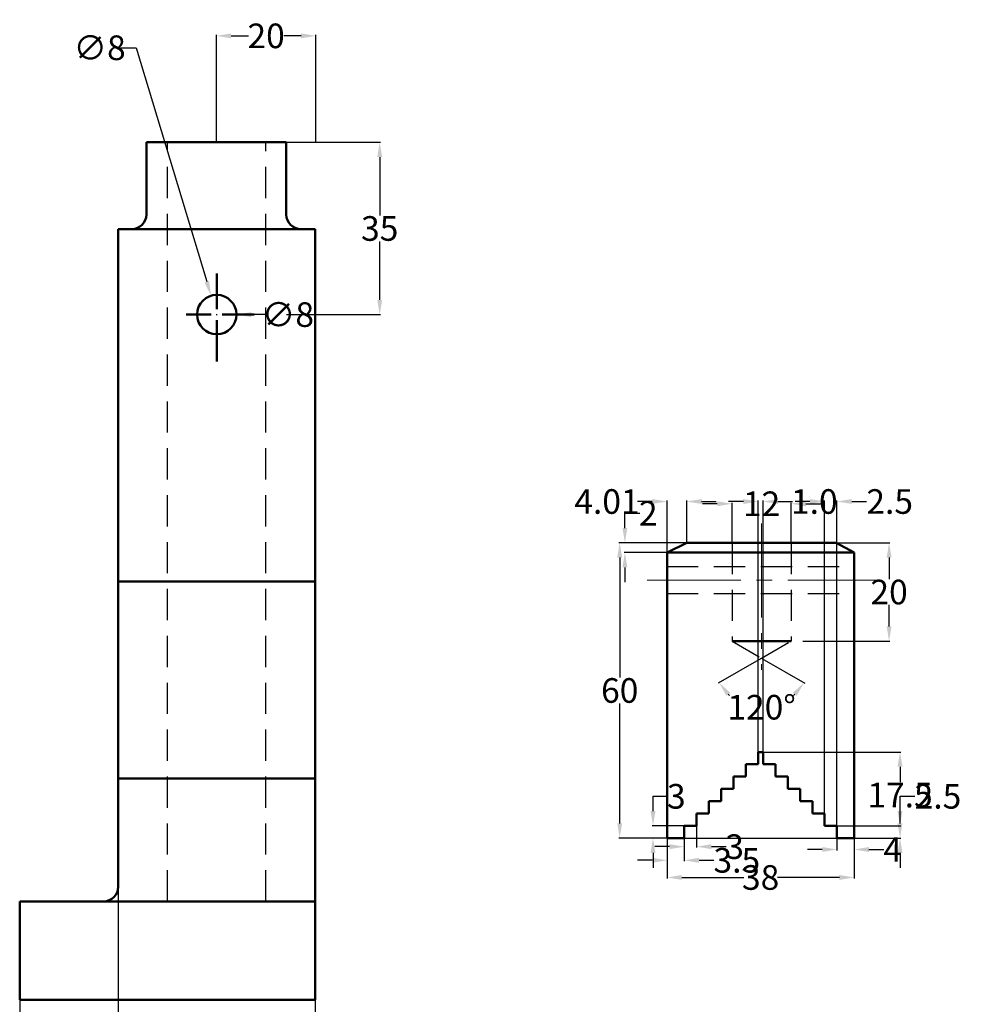
# Model space of a CAD drawing. Units: metres. Extents: x -2793 to -2360, y -31 to 491.
# Tile 4 of 4: x -2552 to -2360, y 144 to 344. Entities that reach past the tile are written whole.
import ezdxf

# ---------------------------------------------------------------- set-up
doc = ezdxf.new("R2010")
doc.units = ezdxf.units.M
doc.linetypes.add('CENTER2', pattern=[28.575, 19.05, -3.175, 3.175, -3.175])
doc.linetypes.add('DASHED2', pattern=[9.525, 6.35, -3.175])
for name, color, linetype, lineweight in [('M-CNTR', 9, 'CENTER2', 18), ('M-DIMS', 2, 'Continuous', 25), ('M-HIDN', 9, 'DASHED2', 25), ('M-OUTL', 7, 'Continuous', 50)]:
    doc.layers.add(name, color=color, linetype=linetype, lineweight=lineweight)
doc.styles.get("Standard").update_dxf_attribs({"font": 'arial.ttf'})
doc.dimstyles.get("Standard").update_dxf_attribs({"dimtxt": 5, "dimasz": 3, "dimexe": 0.18, "dimexo": 0.0625, "dimgap": 0.09, "dimtad": 0, "dimtih": 1, "dimtoh": 1, "dimdec": 0, "dimzin": 0, "dimdsep": 46, "dimtxsty": 'Standard', "dimcen": 0.09, "dimclrd": 254, "dimclre": 254, "dimadec": 0, "dimazin": 0, "dimtfac": 1, "dimtdec": 0, "dimtofl": 0, "dimtmove": 0, "dimatfit": 3, "dimfxl": 1, "dimtolj": 1, "dimtzin": 0, "dimarcsym": 0})

# ---------------------------------------------------------------- blocks, each defined once
blk = doc.blocks.new('*D30')
at = {"layer": 'Defpoints', "color": 0, "transparency": 16777216}
for p in [(-2497.49, 319.4), (-2497.49, 284.4), (-2478.51, 284.4)]:
    blk.add_point(p, dxfattribs=at)
at = {"layer": 'M-DIMS', "color": 0, "lineweight": -2, "transparency": 16777216}
for p, q in [((-2497.43, 319.4), (-2478.33, 319.4)), ((-2478.51, 316.4), (-2478.51, 304.53)), ((-2478.51, 287.4), (-2478.51, 299.27)), ((-2497.43, 284.4), (-2478.33, 284.4))]:
    blk.add_line(p, q, dxfattribs=at)
at = {"layer": 'M-DIMS', "color": 0, "transparency": 16777216}
for points in [[(-2479.01, 316.4), (-2478.01, 316.4), (-2478.51, 319.4)], [(-2479.01, 287.4), (-2478.01, 287.4), (-2478.51, 284.4)]]:
    blk.add_solid(points, dxfattribs=at)
at = {"layer": 'M-DIMS', "color": 0, "transparency": 16777216, "insert": (-2478.51, 301.9), "char_height": 5, "attachment_point": 5}
blk.add_mtext('\\A1;{\\fTimes New Roman|b0|i0|c0|p18;35}', dxfattribs=at)
blk = doc.blocks.new('*D31')
at = {"layer": 'Defpoints', "color": 0, "transparency": 16777216}
for p in [(-2491.47, 341.03), (-2511.68, 319.4), (-2491.47, 319.4)]:
    blk.add_point(p, dxfattribs=at)
at = {"layer": 'M-DIMS', "color": 0, "lineweight": -2, "transparency": 16777216}
for p, q in [((-2511.68, 319.46), (-2511.68, 341.21)), ((-2508.68, 341.03), (-2505.14, 341.03)), ((-2494.47, 341.03), (-2498, 341.03)), ((-2491.47, 319.46), (-2491.47, 341.21))]:
    blk.add_line(p, q, dxfattribs=at)
at = {"layer": 'M-DIMS', "color": 0, "transparency": 16777216}
for points in [[(-2508.68, 341.53), (-2508.68, 340.53), (-2511.68, 341.03)], [(-2494.47, 341.53), (-2494.47, 340.53), (-2491.47, 341.03)]]:
    blk.add_solid(points, dxfattribs=at)
at = {"layer": 'M-DIMS', "color": 0, "transparency": 16777216, "insert": (-2501.57, 341.03), "char_height": 5, "attachment_point": 5}
blk.add_mtext('\\A1;{\\fTimes New Roman|b0|i0|c0|p18;20}', dxfattribs=at)
blk = doc.blocks.new('*D32')
at = {"layer": 'Defpoints', "color": 0, "transparency": 16777216}
for p in [(-2512.76, 288.23), (-2510.45, 280.57)]:
    blk.add_point(p, dxfattribs=at)
at = {"layer": 'M-DIMS', "color": 0, "lineweight": -2, "transparency": 16777216}
for p, q in [((-2531.14, 338.61), (-2527.94, 338.61)), ((-2527.94, 338.61), (-2513.62, 291.1)), ((-2511.7, 284.4), (-2511.52, 284.4)), ((-2511.61, 284.31), (-2511.61, 284.49))]:
    blk.add_line(p, q, dxfattribs=at)
at = {"layer": 'M-DIMS', "color": 0, "transparency": 16777216}
blk.add_solid([(-2513.15, 291.25), (-2514.1, 290.96), (-2512.76, 288.23)], dxfattribs=at)
at = {"layer": 'M-DIMS', "color": 0, "transparency": 16777216, "insert": (-2535.39, 338.61), "char_height": 5, "attachment_point": 5}
blk.add_mtext('\\A1;{\\fTimes New Roman|b0|i0|c0|p18;∅8}', dxfattribs=at)
blk = doc.blocks.new('*D48')
at = {"layer": 'Defpoints', "color": 0, "transparency": 16777216}
for p in [(-2406.98, 218.04), (-2394.98, 218.04), (-2400.98, 214.59), (-2400.98, 214.59), (-2404.39, 205.24)]:
    blk.add_point(p, dxfattribs=at)
at = {"layer": 'M-DIMS', "color": 0, "lineweight": -2, "transparency": 16777216}
for p, q in [((-2401.04, 214.56), (-2409.76, 209.54)), ((-2400.93, 214.56), (-2392.2, 209.54))]:
    blk.add_line(p, q, dxfattribs=at)
for start, end in [(227.2559, 229.3723), (310.6277, 312.7441)]:
    blk.add_arc((-2400.98, 214.59), 9.95, start, end, dxfattribs=at)
at = {"layer": 'M-DIMS', "color": 0, "transparency": 16777216}
for points in [[(-2408.13, 206.97), (-2407.35, 207.59), (-2409.61, 209.63)], [(-2394.62, 207.59), (-2393.84, 206.97), (-2392.36, 209.63)]]:
    blk.add_solid(points, dxfattribs=at)
at = {"layer": 'M-DIMS', "color": 0, "transparency": 16777216, "insert": (-2400.98, 204.64), "char_height": 5, "attachment_point": 5}
blk.add_mtext('\\A1;{\\fTimes New Roman|b0|i0|c0|p18;120°}', dxfattribs=at)
blk = doc.blocks.new('*D49')
at = {"layer": 'Defpoints', "color": 0, "transparency": 16777216}
for p in [(-2392.68, 238.04), (-2392.68, 218.04), (-2375.09, 218.04)]:
    blk.add_point(p, dxfattribs=at)
at = {"layer": 'M-DIMS', "color": 0, "lineweight": -2, "transparency": 16777216}
for p, q in [((-2392.62, 238.04), (-2374.91, 238.04)), ((-2375.09, 235.04), (-2375.09, 230.67)), ((-2375.09, 221.04), (-2375.09, 225.41)), ((-2392.62, 218.04), (-2374.91, 218.04))]:
    blk.add_line(p, q, dxfattribs=at)
at = {"layer": 'M-DIMS', "color": 0, "transparency": 16777216}
for points in [[(-2375.59, 235.04), (-2374.59, 235.04), (-2375.09, 238.04)], [(-2375.59, 221.04), (-2374.59, 221.04), (-2375.09, 218.04)]]:
    blk.add_solid(points, dxfattribs=at)
at = {"layer": 'M-DIMS', "color": 0, "transparency": 16777216, "insert": (-2375.09, 228.04), "char_height": 5, "attachment_point": 5}
blk.add_mtext('\\A1;{\\fTimes New Roman|b0|i0|c0|p18;20}', dxfattribs=at)
blk = doc.blocks.new('*D50')
at = {"layer": 'Defpoints', "color": 0, "transparency": 16777216}
for p in [(-2394.98, 245.97), (-2406.98, 238.04), (-2394.98, 238.04)]:
    blk.add_point(p, dxfattribs=at)
at = {"layer": 'M-DIMS', "color": 0, "lineweight": -2, "transparency": 16777216}
for p, q in [((-2406.98, 238.1), (-2406.98, 246.15)), ((-2394.98, 238.1), (-2394.98, 246.15)), ((-2409.98, 245.97), (-2412.98, 245.97)), ((-2391.98, 245.97), (-2388.98, 245.97))]:
    blk.add_line(p, q, dxfattribs=at)
at = {"layer": 'M-DIMS', "color": 0, "transparency": 16777216}
for points in [[(-2409.98, 246.47), (-2409.98, 245.47), (-2406.98, 245.97)], [(-2391.98, 246.47), (-2391.98, 245.47), (-2394.98, 245.97)]]:
    blk.add_solid(points, dxfattribs=at)
at = {"layer": 'M-DIMS', "color": 0, "transparency": 16777216, "insert": (-2400.98, 245.97), "char_height": 5, "attachment_point": 5}
blk.add_mtext('\\A1;{\\fTimes New Roman|b0|i0|c0|p18;12}', dxfattribs=at)
blk = doc.blocks.new('*D51')
at = {"layer": 'Defpoints', "color": 0, "transparency": 16777216}
for p in [(-2420.83, 238.04), (-2429.78, 178.04), (-2420.17, 178.04)]:
    blk.add_point(p, dxfattribs=at)
at = {"layer": 'M-DIMS', "color": 0, "lineweight": -2, "transparency": 16777216}
for p, q in [((-2420.9, 238.04), (-2429.96, 238.04)), ((-2429.78, 235.04), (-2429.78, 210.67)), ((-2429.78, 181.04), (-2429.78, 205.41)), ((-2420.23, 178.04), (-2429.96, 178.04))]:
    blk.add_line(p, q, dxfattribs=at)
at = {"layer": 'M-DIMS', "color": 0, "transparency": 16777216}
for points in [[(-2430.28, 235.04), (-2429.28, 235.04), (-2429.78, 238.04)], [(-2430.28, 181.04), (-2429.28, 181.04), (-2429.78, 178.04)]]:
    blk.add_solid(points, dxfattribs=at)
at = {"layer": 'M-DIMS', "color": 0, "transparency": 16777216, "insert": (-2429.78, 208.04), "char_height": 5, "attachment_point": 5}
blk.add_mtext('\\A1;{\\fTimes New Roman|b0|i0|c0|p18;60}', dxfattribs=at)
blk = doc.blocks.new('*D52')
at = {"layer": 'Defpoints', "color": 0, "transparency": 16777216}
for p in [(-2423.02, 180.54), (-2416.67, 180.54), (-2416.67, 178.04)]:
    blk.add_point(p, dxfattribs=at)
at = {"layer": 'M-DIMS', "color": 0, "lineweight": -2, "transparency": 16777216}
for p, q in [((-2423.02, 183.54), (-2423.02, 186.54)), ((-2423.02, 186.54), (-2420.02, 186.54)), ((-2416.73, 180.54), (-2423.2, 180.54)), ((-2416.73, 178.04), (-2423.2, 178.04)), ((-2423.02, 175.04), (-2423.02, 172.04))]:
    blk.add_line(p, q, dxfattribs=at)
at = {"layer": 'M-DIMS', "color": 0, "transparency": 16777216}
for points in [[(-2423.52, 183.54), (-2422.52, 183.54), (-2423.02, 180.54)], [(-2423.52, 175.04), (-2422.52, 175.04), (-2423.02, 178.04)]]:
    blk.add_solid(points, dxfattribs=at)
at = {"layer": 'M-DIMS', "color": 0, "transparency": 16777216, "insert": (-2418.29, 186.54), "char_height": 5, "attachment_point": 5}
blk.add_mtext('\\A1;3', dxfattribs=at)
blk = doc.blocks.new('*D53')
at = {"layer": 'Defpoints', "color": 0, "transparency": 16777216}
for p in [(-2416.67, 180.54), (-2414.17, 180.54), (-2414.17, 176.31)]:
    blk.add_point(p, dxfattribs=at)
at = {"layer": 'M-DIMS', "color": 0, "lineweight": -2, "transparency": 16777216}
for p, q in [((-2416.67, 180.48), (-2416.67, 176.13)), ((-2414.17, 180.48), (-2414.17, 176.13)), ((-2419.67, 176.31), (-2422.67, 176.31)), ((-2411.17, 176.31), (-2408.17, 176.31))]:
    blk.add_line(p, q, dxfattribs=at)
at = {"layer": 'M-DIMS', "color": 0, "transparency": 16777216}
for points in [[(-2419.67, 176.81), (-2419.67, 175.81), (-2416.67, 176.31)], [(-2411.17, 176.81), (-2411.17, 175.81), (-2414.17, 176.31)]]:
    blk.add_solid(points, dxfattribs=at)
at = {"layer": 'M-DIMS', "color": 0, "transparency": 16777216, "insert": (-2406.45, 176.31), "char_height": 5, "attachment_point": 5}
blk.add_mtext('\\A1;3', dxfattribs=at)
blk = doc.blocks.new('*D54')
at = {"layer": 'Defpoints', "color": 0, "transparency": 16777216}
for p in [(-2420.17, 178.04), (-2382.17, 178.04), (-2382.17, 170.05)]:
    blk.add_point(p, dxfattribs=at)
at = {"layer": 'M-DIMS', "color": 0, "lineweight": -2, "transparency": 16777216}
for p, q in [((-2420.17, 177.98), (-2420.17, 169.87)), ((-2382.17, 177.98), (-2382.17, 169.87)), ((-2417.17, 170.05), (-2404.59, 170.05)), ((-2385.17, 170.05), (-2397.75, 170.05))]:
    blk.add_line(p, q, dxfattribs=at)
at = {"layer": 'M-DIMS', "color": 0, "transparency": 16777216}
for points in [[(-2417.17, 170.55), (-2417.17, 169.55), (-2420.17, 170.05)], [(-2385.17, 170.55), (-2385.17, 169.55), (-2382.17, 170.05)]]:
    blk.add_solid(points, dxfattribs=at)
at = {"layer": 'M-DIMS', "color": 0, "transparency": 16777216, "insert": (-2401.17, 170.05), "char_height": 5, "attachment_point": 5}
blk.add_mtext('\\A1;{\\fTimes New Roman|b0|i0|c0|p18;38}', dxfattribs=at)
blk = doc.blocks.new('*D55')
at = {"layer": 'Defpoints', "color": 0, "transparency": 16777216}
for p in [(-2385.67, 178.04), (-2382.17, 178.04), (-2382.17, 175.73)]:
    blk.add_point(p, dxfattribs=at)
at = {"layer": 'M-DIMS', "color": 0, "lineweight": -2, "transparency": 16777216}
for p, q in [((-2385.67, 177.98), (-2385.67, 175.55)), ((-2382.17, 177.98), (-2382.17, 175.55)), ((-2388.67, 175.73), (-2391.67, 175.73)), ((-2379.17, 175.73), (-2376.17, 175.73))]:
    blk.add_line(p, q, dxfattribs=at)
at = {"layer": 'M-DIMS', "color": 0, "transparency": 16777216}
for points in [[(-2388.67, 176.23), (-2388.67, 175.23), (-2385.67, 175.73)], [(-2379.17, 176.23), (-2379.17, 175.23), (-2382.17, 175.73)]]:
    blk.add_solid(points, dxfattribs=at)
at = {"layer": 'M-DIMS', "color": 0, "transparency": 16777216, "insert": (-2374.35, 175.73), "char_height": 5, "attachment_point": 5}
blk.add_mtext('\\A1;4', dxfattribs=at)
blk = doc.blocks.new('*D58')
at = {"layer": 'Defpoints', "color": 0, "transparency": 16777216}
for p in [(-2531.61, 168.18), (-2551.61, 165.18), (-2531.61, 121.23)]:
    blk.add_point(p, dxfattribs=at)
at = {"layer": 'M-DIMS', "color": 254, "lineweight": -2, "transparency": 16777216}
for p, q in [((-2531.61, 168.11), (-2531.61, 121.05)), ((-2551.61, 165.11), (-2551.61, 121.05)), ((-2548.61, 121.23), (-2545.31, 121.23)), ((-2534.61, 121.23), (-2537.9, 121.23))]:
    blk.add_line(p, q, dxfattribs=at)
at = {"layer": 'M-DIMS', "color": 254, "transparency": 16777216}
for points in [[(-2548.61, 121.73), (-2548.61, 120.73), (-2551.61, 121.23)], [(-2534.61, 121.73), (-2534.61, 120.73), (-2531.61, 121.23)]]:
    blk.add_solid(points, dxfattribs=at)
at = {"layer": 'M-DIMS', "color": 0, "transparency": 16777216, "insert": (-2541.61, 121.23), "char_height": 5, "attachment_point": 5}
blk.add_mtext('\\A1;20', dxfattribs=at)
blk = doc.blocks.new('*D59')
at = {"layer": 'Defpoints', "color": 0, "transparency": 16777216}
for p in [(-2531.61, 168.18), (-2491.61, 145.18), (-2491.61, 121.23)]:
    blk.add_point(p, dxfattribs=at)
at = {"layer": 'M-DIMS', "color": 254, "lineweight": -2, "transparency": 16777216}
for p, q in [((-2531.61, 168.11), (-2531.61, 121.05)), ((-2491.61, 145.11), (-2491.61, 121.05)), ((-2528.61, 121.23), (-2515.37, 121.23)), ((-2494.61, 121.23), (-2507.84, 121.23))]:
    blk.add_line(p, q, dxfattribs=at)
at = {"layer": 'M-DIMS', "color": 254, "transparency": 16777216}
for points in [[(-2528.61, 121.73), (-2528.61, 120.73), (-2531.61, 121.23)], [(-2494.61, 121.73), (-2494.61, 120.73), (-2491.61, 121.23)]]:
    blk.add_solid(points, dxfattribs=at)
at = {"layer": 'M-DIMS', "color": 0, "transparency": 16777216, "insert": (-2511.61, 121.23), "char_height": 5, "attachment_point": 5}
blk.add_mtext('\\A1;40', dxfattribs=at)
blk = doc.blocks.new('*D60')
at = {"layer": 'Defpoints', "color": 0, "transparency": 16777216}
for p in [(-2420.17, 246.43), (-2416.17, 238.04), (-2420.17, 236.04)]:
    blk.add_point(p, dxfattribs=at)
at = {"layer": 'M-DIMS', "color": 254, "lineweight": -2, "transparency": 16777216}
for p, q in [((-2423.17, 246.43), (-2426.17, 246.43)), ((-2420.17, 236.1), (-2420.17, 246.61)), ((-2416.17, 238.1), (-2416.17, 246.61)), ((-2413.17, 246.43), (-2410.17, 246.43))]:
    blk.add_line(p, q, dxfattribs=at)
at = {"layer": 'M-DIMS', "color": 254, "transparency": 16777216}
for points in [[(-2423.17, 246.93), (-2423.17, 245.93), (-2420.17, 246.43)], [(-2413.17, 246.93), (-2413.17, 245.93), (-2416.17, 246.43)]]:
    blk.add_solid(points, dxfattribs=at)
at = {"layer": 'M-DIMS', "color": 0, "transparency": 16777216, "insert": (-2432.37, 246.43), "char_height": 5, "attachment_point": 5}
blk.add_mtext('\\A1;4.01', dxfattribs=at)
blk = doc.blocks.new('*D61')
at = {"layer": 'Defpoints', "color": 0, "transparency": 16777216}
for p in [(-2428.73, 238.04), (-2416.17, 238.04), (-2420.17, 236.04)]:
    blk.add_point(p, dxfattribs=at)
at = {"layer": 'M-DIMS', "color": 254, "lineweight": -2, "transparency": 16777216}
for p, q in [((-2428.73, 241.04), (-2428.73, 244.04)), ((-2428.73, 244.04), (-2425.73, 244.04)), ((-2416.23, 238.04), (-2428.91, 238.04)), ((-2420.23, 236.04), (-2428.91, 236.04)), ((-2428.73, 233.04), (-2428.73, 230.04))]:
    blk.add_line(p, q, dxfattribs=at)
at = {"layer": 'M-DIMS', "color": 254, "transparency": 16777216}
for points in [[(-2429.23, 241.04), (-2428.23, 241.04), (-2428.73, 238.04)], [(-2429.23, 233.04), (-2428.23, 233.04), (-2428.73, 236.04)]]:
    blk.add_solid(points, dxfattribs=at)
at = {"layer": 'M-DIMS', "color": 0, "transparency": 16777216, "insert": (-2423.98, 244.04), "char_height": 5, "attachment_point": 5}
blk.add_mtext('\\A1;2', dxfattribs=at)
blk = doc.blocks.new('*D62')
at = {"layer": 'Defpoints', "color": 0, "transparency": 16777216}
for p in [(-2401.67, 195.54), (-2372.87, 195.54), (-2420.17, 178.04)]:
    blk.add_point(p, dxfattribs=at)
at = {"layer": 'M-DIMS', "color": 254, "lineweight": -2, "transparency": 16777216}
for p, q in [((-2401.61, 195.54), (-2372.69, 195.54)), ((-2372.87, 192.54), (-2372.87, 189.43)), ((-2372.87, 181.04), (-2372.87, 184.15)), ((-2420.11, 178.04), (-2372.69, 178.04))]:
    blk.add_line(p, q, dxfattribs=at)
at = {"layer": 'M-DIMS', "color": 254, "transparency": 16777216}
for points in [[(-2373.37, 192.54), (-2372.37, 192.54), (-2372.87, 195.54)], [(-2373.37, 181.04), (-2372.37, 181.04), (-2372.87, 178.04)]]:
    blk.add_solid(points, dxfattribs=at)
at = {"layer": 'M-DIMS', "color": 0, "transparency": 16777216, "insert": (-2372.87, 186.79), "char_height": 5, "attachment_point": 5}
blk.add_mtext('\\A1;17.5', dxfattribs=at)
blk = doc.blocks.new('*D69')
at = {"layer": 'Defpoints', "color": 0, "transparency": 16777216}
for p in [(-2515.61, 284.4), (-2507.61, 284.4)]:
    blk.add_point(p, dxfattribs=at)
at = {"layer": 'M-DIMS', "color": 254, "lineweight": -2, "transparency": 16777216}
for p, q in [((-2511.7, 284.4), (-2511.52, 284.4)), ((-2511.61, 284.31), (-2511.61, 284.49)), ((-2501.61, 284.4), (-2504.61, 284.4))]:
    blk.add_line(p, q, dxfattribs=at)
at = {"layer": 'M-DIMS', "color": 254, "transparency": 16777216}
blk.add_solid([(-2504.61, 284.9), (-2504.61, 283.9), (-2507.61, 284.4)], dxfattribs=at)
at = {"layer": 'M-DIMS', "color": 0, "transparency": 16777216, "insert": (-2497.15, 284.4), "char_height": 5, "attachment_point": 5}
blk.add_mtext('\\A1;∅8', dxfattribs=at)
blk = doc.blocks.new('*D70')
at = {"layer": 'Defpoints', "color": 0, "transparency": 16777216}
for p in [(-2385.67, 180.54), (-2372.87, 180.54), (-2385.67, 178.04)]:
    blk.add_point(p, dxfattribs=at)
at = {"layer": 'M-DIMS', "color": 254, "lineweight": -2, "transparency": 16777216}
for p, q in [((-2372.87, 183.54), (-2372.87, 186.54)), ((-2372.87, 186.54), (-2369.87, 186.54)), ((-2385.61, 180.54), (-2372.69, 180.54)), ((-2385.61, 178.04), (-2372.69, 178.04)), ((-2372.87, 175.04), (-2372.87, 172.04))]:
    blk.add_line(p, q, dxfattribs=at)
at = {"layer": 'M-DIMS', "color": 254, "transparency": 16777216}
for points in [[(-2373.37, 183.54), (-2372.37, 183.54), (-2372.87, 180.54)], [(-2373.37, 175.04), (-2372.37, 175.04), (-2372.87, 178.04)]]:
    blk.add_solid(points, dxfattribs=at)
at = {"layer": 'M-DIMS', "color": 0, "transparency": 16777216, "insert": (-2365.16, 186.54), "char_height": 5, "attachment_point": 5}
blk.add_mtext('\\A1;2.5', dxfattribs=at)
blk = doc.blocks.new('*D71')
at = {"layer": 'Defpoints', "color": 0, "transparency": 16777216}
for p in [(-2385.67, 246.43), (-2388.17, 180.54), (-2385.67, 180.54)]:
    blk.add_point(p, dxfattribs=at)
at = {"layer": 'M-DIMS', "color": 254, "lineweight": -2, "transparency": 16777216}
for p, q in [((-2391.17, 246.43), (-2394.17, 246.43)), ((-2388.17, 180.6), (-2388.17, 246.61)), ((-2385.67, 180.6), (-2385.67, 246.61)), ((-2382.67, 246.43), (-2379.67, 246.43))]:
    blk.add_line(p, q, dxfattribs=at)
at = {"layer": 'M-DIMS', "color": 254, "transparency": 16777216}
for points in [[(-2391.17, 246.93), (-2391.17, 245.93), (-2388.17, 246.43)], [(-2382.67, 246.93), (-2382.67, 245.93), (-2385.67, 246.43)]]:
    blk.add_solid(points, dxfattribs=at)
at = {"layer": 'M-DIMS', "color": 0, "transparency": 16777216, "insert": (-2374.97, 246.43), "char_height": 5, "attachment_point": 5}
blk.add_mtext('\\A1;2.5', dxfattribs=at)
blk = doc.blocks.new('*D72')
at = {"layer": 'Defpoints', "color": 0, "transparency": 16777216}
for p in [(-2420.17, 178.04), (-2416.67, 178.04), (-2416.67, 173.54)]:
    blk.add_point(p, dxfattribs=at)
at = {"layer": 'M-DIMS', "color": 254, "lineweight": -2, "transparency": 16777216}
for p, q in [((-2420.17, 177.98), (-2420.17, 173.36)), ((-2416.67, 177.98), (-2416.67, 173.36)), ((-2423.17, 173.54), (-2426.17, 173.54)), ((-2413.67, 173.54), (-2410.67, 173.54))]:
    blk.add_line(p, q, dxfattribs=at)
at = {"layer": 'M-DIMS', "color": 254, "transparency": 16777216}
for points in [[(-2423.17, 174.04), (-2423.17, 173.04), (-2420.17, 173.54)], [(-2413.67, 174.04), (-2413.67, 173.04), (-2416.67, 173.54)]]:
    blk.add_solid(points, dxfattribs=at)
at = {"layer": 'M-DIMS', "color": 0, "transparency": 16777216, "insert": (-2406.01, 173.54), "char_height": 5, "attachment_point": 5}
blk.add_mtext('\\A1;3.5', dxfattribs=at)
blk = doc.blocks.new('*D73')
at = {"layer": 'Defpoints', "color": 0, "transparency": 16777216}
for p in [(-2400.67, 246.43), (-2401.67, 195.54), (-2400.67, 195.54)]:
    blk.add_point(p, dxfattribs=at)
at = {"layer": 'M-DIMS', "color": 254, "lineweight": -2, "transparency": 16777216}
for p, q in [((-2404.67, 246.43), (-2407.67, 246.43)), ((-2401.67, 195.6), (-2401.67, 246.61)), ((-2400.67, 195.6), (-2400.67, 246.61)), ((-2397.67, 246.43), (-2394.67, 246.43))]:
    blk.add_line(p, q, dxfattribs=at)
at = {"layer": 'M-DIMS', "color": 254, "transparency": 16777216}
for points in [[(-2404.67, 246.93), (-2404.67, 245.93), (-2401.67, 246.43)], [(-2397.67, 246.93), (-2397.67, 245.93), (-2400.67, 246.43)]]:
    blk.add_solid(points, dxfattribs=at)
at = {"layer": 'M-DIMS', "color": 0, "transparency": 16777216, "insert": (-2390.27, 246.43), "char_height": 5, "attachment_point": 5}
blk.add_mtext('\\A1;1.0', dxfattribs=at)

msp = doc.modelspace()

# ---------------------------------------------------------------- linework, layer by layer
at = {"layer": 'M-CNTR'}
for p, q in [((-2400.983, 241.93), (-2400.983, 212.207)), ((-2424.228, 230.473), (-2377.365, 230.473))]:
    msp.add_line(p, q, dxfattribs=at)
at = {"layer": 'M-HIDN'}
for p, q in [((-2521.605, 165.175), (-2521.605, 319.401)), ((-2501.605, 165.175), (-2501.605, 319.401)), ((-2406.983, 238.041), (-2406.983, 218.041)), ((-2394.983, 238.041), (-2394.983, 218.041)), ((-2420.172, 233.239), (-2382.172, 233.239)), ((-2420.172, 227.768), (-2382.172, 227.768)), ((-2406.983, 218.041), (-2400.983, 214.589)), ((-2400.983, 214.589), (-2394.983, 218.041))]:
    msp.add_line(p, q, dxfattribs=at)
at = {"layer": 'M-OUTL'}
for p, q in [((-2525.864, 319.401), (-2497.489, 319.401)), ((-2525.864, 304.765), (-2525.864, 319.401)), ((-2497.489, 304.765), (-2497.489, 319.401)), ((-2531.605, 168.175), (-2531.605, 301.765)), ((-2531.605, 301.765), (-2528.864, 301.765)), ((-2528.864, 301.765), (-2494.489, 301.765)), ((-2494.489, 301.765), (-2491.605, 301.765)), ((-2491.605, 165.175), (-2491.605, 301.765)), ((-2511.605, 285.539), (-2511.605, 292.73)), ((-2517.804, 284.401), (-2512.743, 284.401)), ((-2510.467, 284.401), (-2504.002, 284.401)), ((-2511.605, 274.906), (-2511.605, 283.263)), ((-2420.172, 236.041), (-2416.167, 238.041)), ((-2416.167, 238.041), (-2385.834, 238.041)), ((-2382.172, 236.041), (-2385.834, 238.041)), ((-2420.172, 178.041), (-2420.172, 236.041)), ((-2420.172, 236.041), (-2382.172, 236.041)), ((-2382.172, 236.041), (-2382.172, 178.041)), ((-2531.605, 230.175), (-2491.605, 230.175)), ((-2406.983, 218.041), (-2394.983, 218.041)), ((-2401.672, 193.041), (-2401.672, 195.541)), ((-2400.672, 195.541), (-2401.672, 195.541)), ((-2400.672, 195.541), (-2400.672, 193.041)), ((-2404.172, 190.541), (-2404.172, 193.041)), ((-2401.672, 193.041), (-2404.172, 193.041)), ((-2398.172, 193.041), (-2400.672, 193.041)), ((-2398.172, 193.041), (-2398.172, 190.541)), ((-2531.605, 190.175), (-2491.605, 190.175)), ((-2406.672, 188.041), (-2406.672, 190.541)), ((-2404.172, 190.541), (-2406.672, 190.541)), ((-2395.672, 190.541), (-2398.172, 190.541)), ((-2395.672, 190.541), (-2395.672, 188.041)), ((-2409.172, 185.541), (-2409.172, 188.041)), ((-2406.672, 188.041), (-2409.172, 188.041)), ((-2393.172, 188.041), (-2395.672, 188.041)), ((-2393.172, 188.041), (-2393.172, 185.541)), ((-2411.672, 183.041), (-2411.672, 185.541)), ((-2409.172, 185.541), (-2411.672, 185.541)), ((-2390.672, 185.541), (-2393.172, 185.541)), ((-2390.672, 185.541), (-2390.672, 183.041)), ((-2414.172, 180.541), (-2414.172, 183.041)), ((-2411.672, 183.041), (-2414.172, 183.041)), ((-2388.172, 183.041), (-2390.672, 183.041)), ((-2388.172, 183.041), (-2388.172, 180.541)), ((-2416.672, 178.041), (-2416.672, 180.541)), ((-2414.172, 180.541), (-2416.672, 180.541)), ((-2385.672, 180.541), (-2388.172, 180.541)), ((-2385.672, 180.541), (-2385.672, 178.041)), ((-2416.672, 178.041), (-2420.172, 178.041)), ((-2382.172, 178.041), (-2385.672, 178.041)), ((-2534.605, 165.175), (-2551.605, 165.175)), ((-2551.605, 165.175), (-2551.605, 145.175)), ((-2534.605, 165.175), (-2491.605, 165.175)), ((-2491.605, 145.175), (-2491.605, 165.175)), ((-2551.605, 145.175), (-2491.605, 145.175))]:
    msp.add_line(p, q, dxfattribs=at)
msp.add_circle((-2511.605, 284.401), 4, dxfattribs=at)
for centre, start, end in [((-2528.864, 304.765), 270, 360), ((-2494.489, 304.765), 180, 270), ((-2534.605, 168.175), 270, 0)]:
    msp.add_arc(centre, 3, start, end, dxfattribs=at)

# ---------------------------------------------------------------- dimensions: what is measured, and where the dimension line sits
at = {"layer": 'M-DIMS'}
for base, p1, p2, picture, middle in [((-2491.472, 341.033), (-2511.676, 319.401), (-2491.472, 319.401), '*D31', (-2501.574, 341.033)), ((-2394.983, 245.973), (-2406.983, 238.041), (-2394.983, 238.041), '*D50', (-2400.983, 245.973)), ((-2382.172, 170.047), (-2420.172, 178.041), (-2382.172, 178.041), '*D54', (-2401.172, 170.047))]:
    dim = msp.add_linear_dim(base=base, p1=p1, p2=p2, text='{\\fTimes New Roman|b0|i0|c0|p18;<>}', dimstyle='Standard', override={"dimclrd": 0, "dimclre": 0, "dimclrt": 0}, dxfattribs=at)
    dim.commit()
    dim.dimension.update_dxf_attribs({"geometry": picture, "text_midpoint": middle})
dim = msp.add_diameter_dim_2p(p1=(-2510.451, 280.571), p2=(-2512.759, 288.231), text='{\\fTimes New Roman|b0|i0|c0|p18;<>}', dimstyle='Standard', override={"dimclrd": 0, "dimclre": 0, "dimclrt": 0}, dxfattribs=at)
dim.commit()
dim.dimension.update_dxf_attribs({"geometry": '*D32', "text_midpoint": (-2535.392, 338.609), "dimtype": 163})
for base, p1, p2, picture, middle in [((-2478.509, 284.401), (-2497.489, 319.401), (-2497.489, 284.401), '*D30', (-2478.509, 301.901)), ((-2429.776, 178.041), (-2420.834, 238.041), (-2420.172, 178.041), '*D51', (-2429.776, 208.041)), ((-2375.092, 218.041), (-2392.684, 238.041), (-2392.684, 218.041), '*D49', (-2375.092, 228.041))]:
    dim = msp.add_linear_dim(base=base, p1=p1, p2=p2, angle=90, text='{\\fTimes New Roman|b0|i0|c0|p18;<>}', dimstyle='Standard', override={"dimclrd": 0, "dimclre": 0, "dimclrt": 0}, dxfattribs=at)
    dim.commit()
    dim.dimension.update_dxf_attribs({"geometry": picture, "text_midpoint": middle})
dim = msp.add_diameter_dim_2p(p1=(-2515.605, 284.402), p2=(-2507.605, 284.4), dimstyle='Standard', override={"dimdec": 0, "dimlfac": 1, "dimrnd": 0, "dimzin": 0, "dimdsep": 46, "dimlunit": 2}, dxfattribs=at)
dim.commit()
dim.dimension.update_dxf_attribs({"geometry": '*D69', "text_midpoint": (-2501.605, 284.398), "dimtype": 163})
for base, p1, p2, override, picture, middle in [((-2420.1725, 246.4295), (-2416.167, 238.041), (-2420.1725, 236.041), {"dimdec": 2, "dimlfac": 1, "dimrnd": 0, "dimzin": 0, "dimdsep": 46, "dimlunit": 2}, '*D60', (-2432.3744, 246.4295)), ((-2400.672, 246.43), (-2401.672, 195.541), (-2400.672, 195.541), {"dimdec": 1, "dimlfac": 1, "dimrnd": 0, "dimzin": 0, "dimdsep": 46, "dimlunit": 2}, '*D73', (-2390.275, 246.43)), ((-2385.672, 246.43), (-2388.172, 180.541), (-2385.672, 180.541), {"dimdec": 1, "dimlfac": 1, "dimrnd": 0, "dimzin": 0, "dimdsep": 46, "dimlunit": 2}, '*D71', (-2374.97, 246.43)), ((-2414.17249576, 176.307811769), (-2416.67249576, 180.541027027), (-2414.17249576, 180.541027027), {"dimclrd": 0, "dimclre": 0, "dimclrt": 0}, '*D53', (-2406.445387983, 176.307811769)), ((-2416.672, 173.541), (-2420.172, 178.041), (-2416.672, 178.041), {"dimdec": 1, "dimlfac": 1, "dimrnd": 0, "dimzin": 0, "dimdsep": 46, "dimlunit": 2}, '*D72', (-2406.014, 173.541)), ((-2382.17249576, 175.732744734), (-2385.67249576, 178.041027027), (-2382.17249576, 178.041027027), {"dimclrd": 0, "dimclre": 0, "dimclrt": 0}, '*D55', (-2374.353300671, 175.732744734)), ((-2531.605, 121.229), (-2551.605, 165.175), (-2531.605, 168.175), {"dimdec": 0, "dimlfac": 1, "dimrnd": 0, "dimzin": 0, "dimdsep": 46, "dimlunit": 2}, '*D58', (-2541.605, 121.229)), ((-2491.605, 121.229), (-2531.605, 168.175), (-2491.605, 145.175), {"dimdec": 0, "dimlfac": 1, "dimrnd": 0, "dimzin": 0, "dimdsep": 46, "dimlunit": 2}, '*D59', (-2511.605, 121.229))]:
    dim = msp.add_linear_dim(base=base, p1=p1, p2=p2, dimstyle='Standard', override=override, dxfattribs=at)
    dim.commit()
    dim.dimension.update_dxf_attribs({"geometry": picture, "text_midpoint": middle})
for base, p1, p2, override, picture, middle in [((-2428.728, 238.041), (-2420.172, 236.041), (-2416.167, 238.041), {"dimdec": 0, "dimlfac": 1, "dimrnd": 0, "dimzin": 0, "dimdsep": 46, "dimlunit": 2}, '*D61', (-2423.982, 244.041)), ((-2372.865, 195.541), (-2420.172, 178.041), (-2401.672, 195.541), {"dimdec": 1, "dimlfac": 1, "dimrnd": 0, "dimzin": 0, "dimdsep": 46, "dimlunit": 2}, '*D62', (-2372.865, 186.791)), ((-2423.017030081, 180.541027027), (-2416.67249576, 178.041027027), (-2416.67249576, 180.541027027), {"dimclrd": 0, "dimclre": 0, "dimclrt": 0}, '*D52', (-2418.289922304, 186.541027027)), ((-2372.865, 180.541), (-2385.672, 178.041), (-2385.672, 180.541), {"dimdec": 1, "dimlfac": 1, "dimrnd": 0, "dimzin": 0, "dimdsep": 46, "dimlunit": 2}, '*D70', (-2365.162, 186.541))]:
    dim = msp.add_linear_dim(base=base, p1=p1, p2=p2, angle=90, dimstyle='Standard', override=override, dxfattribs=at)
    dim.commit()
    dim.dimension.update_dxf_attribs({"geometry": picture, "text_midpoint": middle})
dim = msp.add_angular_dim_2l(base=(-2404.391, 205.239), line1=((-2400.983, 214.589), (-2394.983, 218.041)), line2=((-2406.983, 218.041), (-2400.983, 214.589)), text='{\\fTimes New Roman|b0|i0|c0|p18;<>}', dimstyle='Standard', override={"dimclrd": 0, "dimclre": 0, "dimclrt": 0}, dxfattribs=at)
dim.commit()
dim.dimension.update_dxf_attribs({"geometry": '*D48', "text_midpoint": (-2400.983, 204.637)})

doc.saveas('drawing.dxf')
